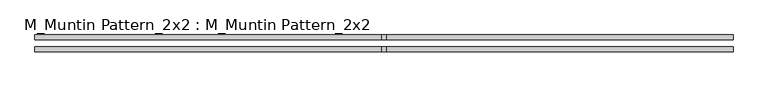
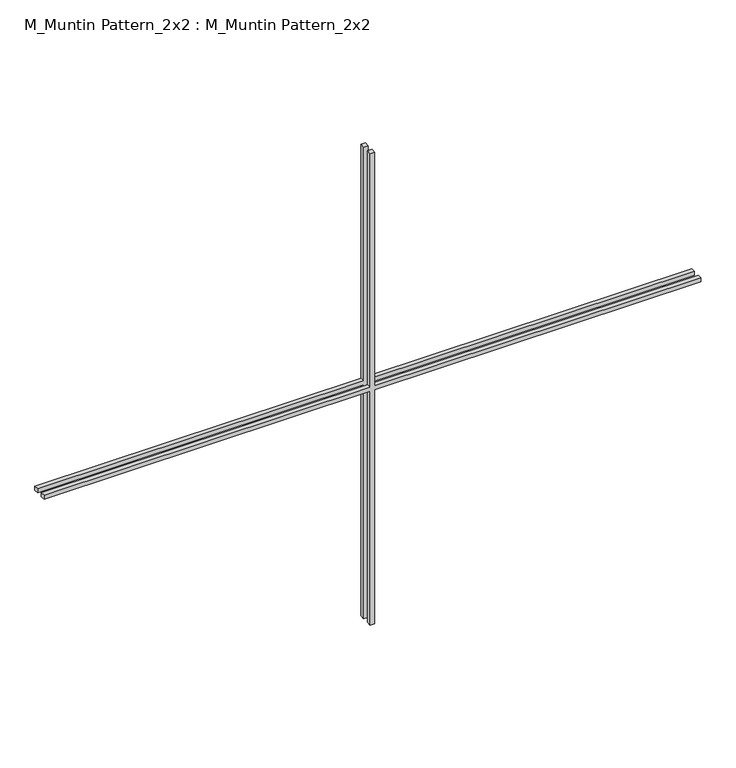
"""IFC4 building model written with IfcOpenShell, lengths in millimetres: proxy geometry, M_Muntin Pattern_2x2 : M_Muntin Pattern_2x2."""

from ifc_helpers import new_model, si_unit, frame, origin, place, context, project, spatial, polyline, outline, extrude, source, transform, mapped, element, save


def m_muntin_pattern_2x2_m_muntin_pattern_2x2_665a5da2(model_context):
    return source(origin(), model_context, "Body", "SweptSolid", [
        extrude(outline(polyline([(707.1375, -6.35), (707.1375, -923.8), (694.4375, -923.8), (694.4375, -6.35), (0.0, -6.35), (0.0, 6.35), (694.4375, 6.35), (694.4375, 923.8), (707.1375, 923.8), (707.1375, 6.35), (1401.575, 6.35), (1401.575, -6.35), (707.1375, -6.35)])), frame((0.0, 9.525, 0.0), z_axis=(0.0, 1.0, 0.0), x_axis=(0.0, 0.0, 1.0)), (0.0, 0.0, 1.0), 12.7),
        extrude(outline(polyline([(707.1375, -6.35), (707.1375, -923.8), (694.4375, -923.8), (694.4375, -6.35), (0.0, -6.35), (0.0, 6.35), (694.4375, 6.35), (694.4375, 923.8), (707.1375, 923.8), (707.1375, 6.35), (1401.575, 6.35), (1401.575, -6.35), (707.1375, -6.35)])), frame((0.0, -22.225, 0.0), z_axis=(0.0, 1.0, 0.0), x_axis=(0.0, 0.0, 1.0)), (0.0, 0.0, 1.0), 12.7),
    ])


if __name__ == "__main__":
    model = new_model("IFC4")
    model_context = context("Model", 3, world=origin())
    ifc_project = project(units=[si_unit("LENGTHUNIT", "METRE", prefix="MILLI")], contexts=[model_context])
    site = spatial("IfcSite", under=ifc_project)
    building = spatial("IfcBuilding", under=site)
    placement = place(None, origin())
    m_muntin_pattern_2x2_m_muntin_pattern_2x2_shape = m_muntin_pattern_2x2_m_muntin_pattern_2x2_665a5da2(model_context)
    element("IfcBuildingElementProxy", 1, Name="M_Muntin Pattern_2x2 : M_Muntin Pattern_2x2", ObjectType="M_Muntin Pattern_2x2 : M_Muntin Pattern_2x2", at=placement, inside=building, context=model_context, shape_type="MappedRepresentation", body=[
        mapped(m_muntin_pattern_2x2_m_muntin_pattern_2x2_shape, transform((0.0, 0.0, 0.0), x_axis=(1.0, 0.0, 0.0), y_axis=(0.0, 1.0, 0.0), z_axis=(0.0, 0.0, 1.0))),
    ])
    save(model, "model.ifc")

# Revit data of these elements
# Type "M_Muntin Pattern_2x2 : M_Muntin Pattern_2x2"
#   Width [instance default] = 1200 mm
#   Thickness = 12.7 mm
#   Height [instance default] = 1200 mm
#   Distance = 19.05 mm
#   Interior Material [instance default] = none
#   Exterior Material [instance default] = none
#   Default Elevation = 0
# Element 1 (IfcBuildingElementProxy, "M_Muntin Pattern_2x2 : M_Muntin Pattern_2x2")
#   Width = 1847.6 mm
#   Height = 1401.575 mm
#   Interior Material = Wood - Stained
#   Exterior Material = Clad - White
#   Materials on its faces: "Clad - White", "Wood - Stained"
# Materials
#   "Clad - White": class "Wood", colour RGB 242 242 238, transparency 0, Cost = 0
#   "Wood - Stained": class "Wood", colour RGB 224 178 126, transparency 0, Cost = 0
